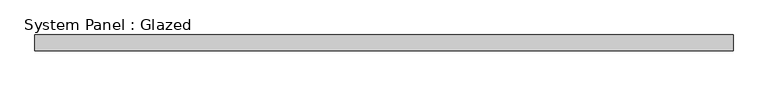
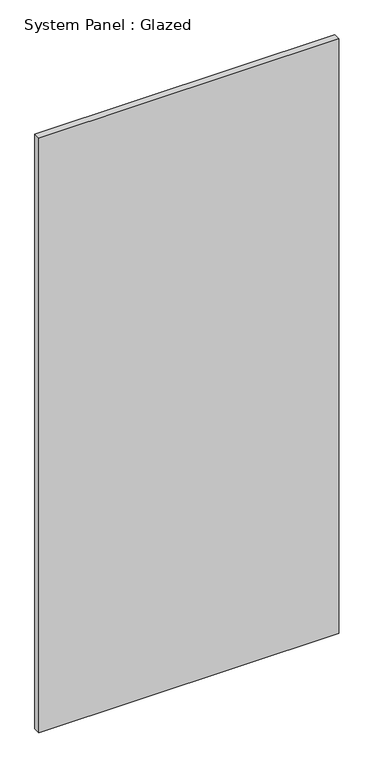
"""IFC4 building model written with IfcOpenShell, lengths in millimetres: plate geometry, System Panel : Glazed."""

from ifc_helpers import new_model, si_unit, origin, origin_with_axes, place, context, project, spatial, polyline, outline, extrude, source, transform, mapped, element, save


def system_panel_glazed_dcfdf68f(model_context):
    return source(origin(), model_context, "Body", "SweptSolid", [
        extrude(outline(polyline([(558.7999999, 19.05), (-558.7999999, 19.05), (-558.7999999, 44.45), (558.7999999, 44.45), (558.7999999, 19.05)])), origin_with_axes(), (0.0, 0.0, 1.0), 2343.15),
    ])


if __name__ == "__main__":
    model = new_model("IFC4")
    model_context = context("Model", 3, world=origin())
    ifc_project = project(units=[si_unit("LENGTHUNIT", "METRE", prefix="MILLI")], contexts=[model_context])
    site = spatial("IfcSite", under=ifc_project)
    building = spatial("IfcBuilding", under=site)
    placement = place(None, origin())
    system_panel_glazed_shape = system_panel_glazed_dcfdf68f(model_context)
    element("IfcPlate", 1, ObjectType="System Panel : Glazed", at=placement, inside=building, context=model_context, shape_type="MappedRepresentation", body=[
        mapped(system_panel_glazed_shape, transform((0.0, 0.0, 0.0), x_axis=(1.0, 0.0, 0.0), y_axis=(0.0, 1.0, 0.0), z_axis=(0.0, 0.0, 1.0))),
    ])
    save(model, "model.ifc")

# Revit data of these elements
# Type "System Panel : Glazed"
#   Construction Type Id = "GSP4R"
#   Analytic Construction = "1/8 in Pilkington single glazing"
#   Visual Light Transmittance = 0.9
#   Solar Heat Gain Coefficient = 0.86
#   Heat Transfer Coefficient (U) = 1.18115 BTU/(h·ft²·°F)
#   Define Thermal Properties by = 1
# Element 1 (IfcPlate, "System Panel : Glazed")
#   Materials on its faces: "Glass"
# Materials
#   "Glass": class "Glass", colour RGB 0 128 192, transparency 0.75, Description = "Soda Lime Glass", Cost = 0
